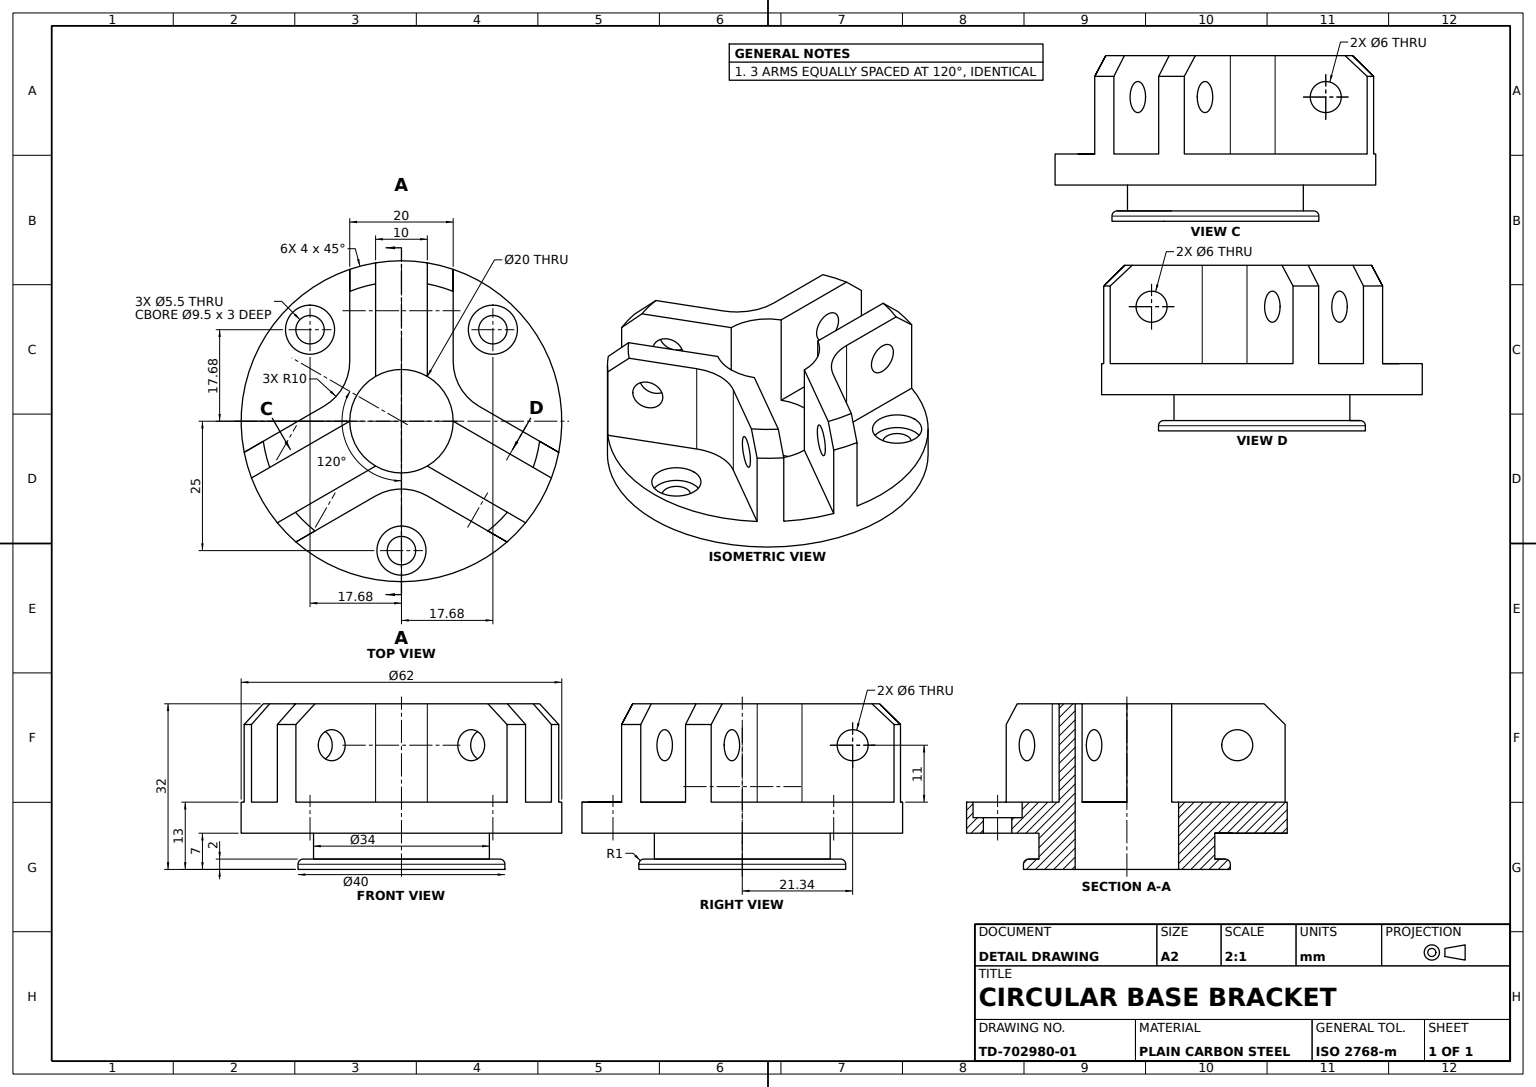
from build123d import *

# Parameters (mm, degrees)
THREE_START                       = 19
THREE_ARMS_DEPTH                  = 19
CENTRE_BORE_SKETCH_R              = 10
CENTRE_BORE_DEPTH                 = 79
ARM_FILLETS_R10_A_R               = 10
ARM_FILLETS_R10_B_R               = 10
ARM_HOLE_1_SKETCH_R               = 3
ARM_HOLE_1_DEPTH                  = 79
ARM_HOLE_2_SKETCH_R               = 3
ARM_HOLE_2_DEPTH                  = 79
ARM_HOLE_3_SKETCH_R               = 3
ARM_HOLE_3_DEPTH                  = 79
ARM_CHAMFER_4MM_SIZE              = 4
BASE_C_BORE_HOLES_5_5_D           = 5.5
BASE_C_BORE_HOLES_5_5_DEPTH       = 9
BASE_C_BORE_HOLES_5_5_CBORE_D     = 9.5
BASE_C_BORE_HOLES_5_5_CBORE_DEPTH = 3


with BuildPart() as part:
    # Base Hub Profile → Base Hub (revolve)
    with BuildSketch(Plane.XY, mode=Mode.PRIVATE) as base_hub_sk:
        with BuildLine():
            Line((0, 0), (-20, 0))
            Line((-20, 0), (-20, 1))
            ThreePointArc((-20, 1), (-19.707106781, 1.707106781), (-19, 2))
            Line((-19, 2), (-17, 2))
            Line((-17, 2), (-17, 7))
            Line((-17, 7), (-31, 7))
            Line((-31, 7), (-31, 13))
            Line((-31, 13), (0, 13))
            Line((0, 13), (0, 0))
        make_face()
    revolve(base_hub_sk.sketch.rotate(Axis((0, 0, 0), (0, 1, 0)), 270), axis=Axis((0, 0, 0), (0, 1, 0)))

    # Arms Profile → Three Arms (add)
    with BuildSketch(Plane(origin=(0, 13, 0), x_dir=(1, 0, 0), z_dir=(0, 1, 0)).offset(THREE_START)):
        with BuildLine():
            Line((-5, 30.594117082), (-5, 2.886751274))
            Line((-5, 2.886751274), (-28.995282363, -10.966932145))
            ThreePointArc((-28.995282363, -10.966932145), (-29.806621866, -8.518526455), (-30.41161139, -6.011147367))
            Line((-30.41161139, -6.011147367), (-10, 5.773502549))
            Line((-10, 5.773502549), (-10, 29.342801502))
            ThreePointArc((-10, 29.342801502), (-7.526051267, 30.072554802), (-5, 30.594117082))
        make_face()
        with BuildLine():
            Line((5, 30.594117082), (5, 2.886751274))
            Line((5, 2.886751274), (28.995282363, -10.966932145))
            ThreePointArc((28.995282363, -10.966932145), (29.806621866, -8.518526455), (30.41161139, -6.011147367))
            Line((30.41161139, -6.011147367), (10, 5.773502549))
            Line((10, 5.773502549), (10, 29.342801502))
            ThreePointArc((10, 29.342801502), (7.526051267, 30.072554802), (5, 30.594117082))
        make_face()
        with BuildLine():
            Line((23.995282177, -19.627186076), (0, -5.773502764))
            Line((0, -5.773502764), (-23.995282177, -19.627186076))
            ThreePointArc((-23.995282177, -19.627186076), (-22.280570319, -21.554029467), (-20.411611017, -23.331655228))
            Line((-20.411611017, -23.331655228), (0, -11.547005527))
            Line((0, -11.547005527), (20.411611017, -23.331655228))
            ThreePointArc((20.411611017, -23.331655228), (22.280570319, -21.554029467), (23.995282177, -19.627186076))
        make_face()
    extrude(amount=-THREE_ARMS_DEPTH)

    # Centre Bore Sketch → Centre Bore (cut)
    with BuildSketch(Plane.XZ):
        with Locations(Location((0, 0, 0), (0, 0, 270))):
            Circle(CENTRE_BORE_SKETCH_R)
    extrude(amount=-CENTRE_BORE_DEPTH, mode=Mode.SUBTRACT)

    # Arm Fillets R10 A
    arm_fillets_r10_a_edges = [part.edges().sort_by_distance(p)[0] for p in [
        (-10, 22.5, -5.773502549),
    ]]
    fillet(arm_fillets_r10_a_edges, radius=ARM_FILLETS_R10_A_R)

    # Arm Fillets R10 B
    arm_fillets_r10_b_edges = [part.edges().sort_by_distance(p)[0] for p in [
        (0, 22.5, 11.547005527),
        (10, 22.5, -5.773502549),
    ]]
    fillet(arm_fillets_r10_b_edges, radius=ARM_FILLETS_R10_B_R)

    # Arm Hole 1 Sketch → Arm Hole 1 (cut)
    with BuildSketch(Plane(origin=(5.000000186, 0, 8.66025393), x_dir=(0.8660253930337038, 0, -0.5000000186208186), z_dir=(0.5000000186208186, 0, 0.8660253930337038))):
        with Locations((-21.342801502, 24)):
            Circle(ARM_HOLE_1_SKETCH_R)
    extrude(amount=-ARM_HOLE_1_DEPTH, mode=Mode.SUBTRACT)

    # Arm Hole 2 Sketch → Arm Hole 2 (cut)
    with BuildSketch(Plane.ZY.offset(10)):
        with Locations((-21.342801502, 24)):
            Circle(ARM_HOLE_2_SKETCH_R)
    extrude(amount=-ARM_HOLE_2_DEPTH, mode=Mode.SUBTRACT)

    # Arm Hole 3 Sketch → Arm Hole 3 (cut)
    with BuildSketch(Plane(origin=(5.000000186, 0, -8.66025393), x_dir=(-0.866025393033704, 0, -0.5000000186208184), z_dir=(0.5000000186208183, 0, -0.8660253930337038))):
        with Locations((-21.342801502, 24)):
            Circle(ARM_HOLE_3_SKETCH_R)
    extrude(amount=-ARM_HOLE_3_DEPTH, mode=Mode.SUBTRACT)

    # Arm Chamfer 4mm
    arm_chamfer_4mm_edges = [part.edges().sort_by_distance(p)[0] for p in [
        (-7.526051267, 32, -30.072554802),
        (-29.806621866, 32, 8.518526455),
        (-22.280570319, 32, 21.554029467),
        (22.280570319, 32, 21.554029467),
        (7.526051267, 32, -30.072554802),
        (29.806621866, 32, 8.518526455),
    ]]
    chamfer(arm_chamfer_4mm_edges, length=ARM_CHAMFER_4MM_SIZE)

    # Base C-Bore Holes Ø5.5
    with Locations(Plane(origin=(0, 13, 0), x_dir=(1, 0, 0), z_dir=(0, 1, 0))):
        with Locations((-17.67766953, 17.67766953), (0, -25), (17.67766953, 17.67766953)):
            CounterBoreHole(BASE_C_BORE_HOLES_5_5_D / 2, BASE_C_BORE_HOLES_5_5_CBORE_D / 2, BASE_C_BORE_HOLES_5_5_CBORE_DEPTH, depth=BASE_C_BORE_HOLES_5_5_DEPTH)


solid = part.part
